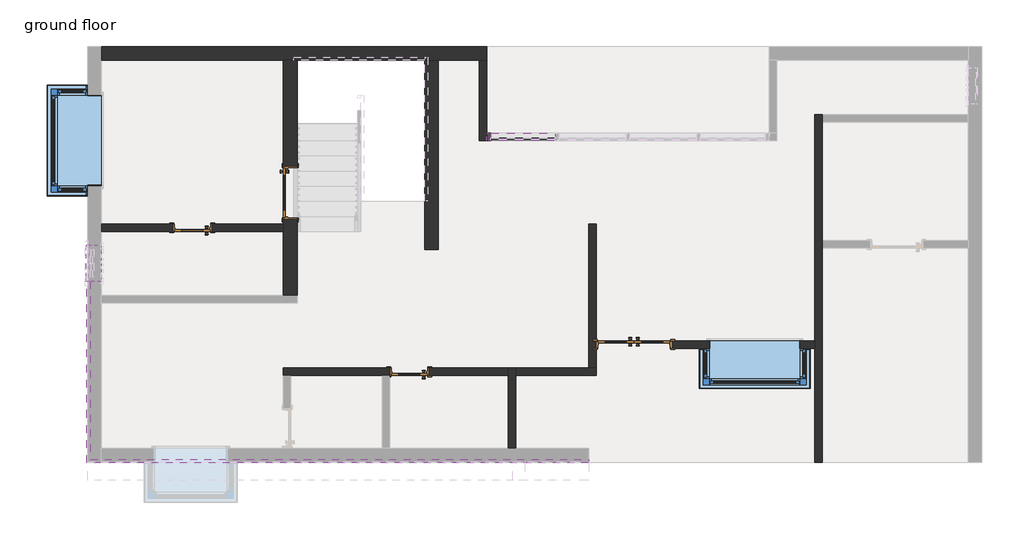
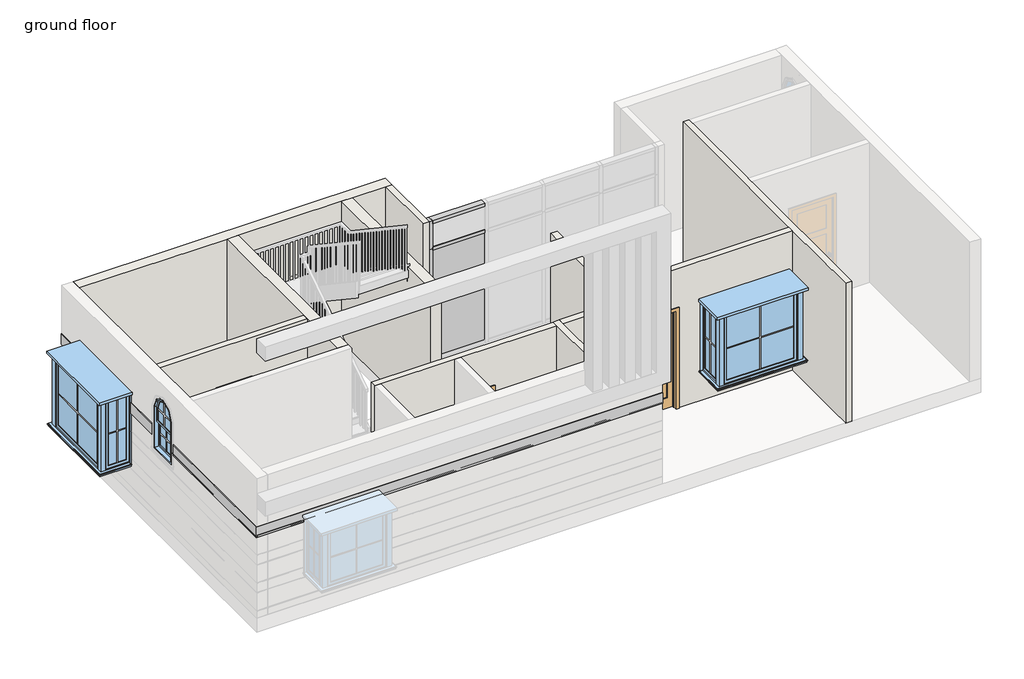
# One storey, part 3 of 5: 11 walls, 4 doors, 4 members, 3 windows, 1 plate, 1 proxy.
"""IFC4 building model written with IfcOpenShell, lengths in millimetres."""

from ifc_helpers import new_model, si_unit, frame, origin, place, context, project, spatial, polyline, circle_curve, ellipse_curve, outline, extrude, faceted_brep, transform, mapped, element, save
from ifc_brep_helpers import plane_surface, cylinder_surface, revolved_surface, advanced_brep
from components import door_interior_double_full_glass_wood_double_door_4_x_7_060eee9d, door_596d7c92, door_5abea521, member_ee409385, member_47bfaf8a, member_5474ae84, member_0cc0e230, system_panel_glazed_91cb7ab6, window_153fc52c, window_dda79932, window_777a1d98

model = new_model("IFC4")

# Units and contexts
model_context = context("Model", 3, world=origin())
ifc_project = project(units=[si_unit("LENGTHUNIT", "METRE", prefix="MILLI")], contexts=[model_context])

# Site, building, storey
site = spatial("IfcSite", under=ifc_project)
building = spatial("IfcBuilding", under=site)
storey = spatial("IfcBuildingStorey", under=building, Name="ground floor", Elevation=304.8)

# Proxy
placement = place(None, origin())
element("IfcBuildingElementProxy", 1, Name="Reveal", ObjectType="Reveal", at=placement, inside=storey, context=model_context, shape_type="AdvancedBrep", body=[
    advanced_brep(
    [(-13193.9516301, -7280.1146427, 2298.7), (-13130.7056301, -7216.8686427, 2298.7), (-13130.7056301, -7216.8686427, 2297.3203242), (-13135.0884393, -7221.2514519, 2292.1465897), (-13158.7091301, -7244.8721427, 2288.2098), (-13177.9470117, -7264.1100243, 2285.00348), (-13186.7126301, -7272.8756427, 2274.656011), (-13186.7126301, -7272.8756427, 2094.143989), (-13177.9470117, -7264.1100243, 2083.79652), (-13158.7091301, -7244.8721427, 2080.5902), (-13135.0884393, -7221.2514519, 2076.6534103), (-13130.7056301, -7216.8686427, 2071.4796758), (-13130.7056301, -7216.8686427, 2070.1), (-13193.9516301, -7280.1146427, 2070.1), (-4797.0672301, -7280.1146427, 2298.7), (-4797.0672301, -7280.1146427, 2070.1), (-4797.0672301, -7216.8686427, 2070.1), (-4797.0672301, -7216.8686427, 2071.4796758), (-4797.0672301, -7221.2514519, 2076.6534103), (-4797.0672301, -7244.8721427, 2080.5902), (-4797.0672301, -7264.1100243, 2083.79652), (-4797.0672301, -7272.8756427, 2094.143989), (-4797.0672301, -7272.8756427, 2274.656011), (-4797.0672301, -7264.1100243, 2285.00348), (-4797.0672301, -7244.8721427, 2288.2098), (-4797.0672301, -7221.2514519, 2292.1465897), (-4797.0672301, -7216.8686427, 2297.3203242), (-4797.0672301, -7216.8686427, 2298.7)],
    [
        (0, 1),
        (1, 2),
        (2, 3, ellipse_curve(frame((-13135.9507301, -7222.1137427, 2297.3203242), z_axis=(-0.7071067811865476, 0.7071067811865476, 0.0), x_axis=(-0.7071067811865475, -0.7071067811865476, 0.0)), 7.4176916, 5.2451)),
        (3, 4),
        (4, 5),
        (5, 6, ellipse_curve(frame((-13176.2224301, -7262.3854427, 2274.656011), z_axis=(0.7071067811865476, -0.7071067811865476, 0.0), x_axis=(0.7071067811865475, 0.7071067811865476, 0.0)), 14.8353831, 10.4902)),
        (6, 7),
        (7, 8, ellipse_curve(frame((-13176.2224301, -7262.3854427, 2094.143989), z_axis=(0.7071067811865476, -0.7071067811865476, 0.0), x_axis=(0.7071067811865475, 0.7071067811865476, 0.0)), 14.8353831, 10.4902)),
        (8, 9),
        (9, 10),
        (10, 11, ellipse_curve(frame((-13135.9507301, -7222.1137427, 2071.4796758), z_axis=(-0.7071067811865476, 0.7071067811865476, 0.0), x_axis=(-0.7071067811865475, -0.7071067811865476, 0.0)), 7.4176916, 5.2451)),
        (11, 12),
        (12, 13),
        (13, 0),
        (14, 15),
        (15, 16),
        (16, 17),
        (17, 18, circle_curve(frame((-4797.0672301, -7222.1137427, 2071.4796758), z_axis=(1.0, 0.0, 0.0), x_axis=(0.0, 1.0, 0.0)), 5.2451)),
        (18, 19),
        (19, 20),
        (20, 21, circle_curve(frame((-4797.0672301, -7262.3854427, 2094.143989), z_axis=(-1.0, 0.0, 0.0), x_axis=(0.0, 1.0, 0.0)), 10.4902)),
        (21, 22),
        (22, 23, circle_curve(frame((-4797.0672301, -7262.3854427, 2274.656011), z_axis=(-1.0, 0.0, 0.0), x_axis=(0.0, 1.0, 0.0)), 10.4902)),
        (23, 24),
        (24, 25),
        (25, 26, circle_curve(frame((-4797.0672301, -7222.1137427, 2297.3203242), z_axis=(1.0, 0.0, 0.0), x_axis=(0.0, 1.0, 0.0)), 5.2451)),
        (26, 27),
        (27, 14),
        (0, 14),
        (27, 1),
        (26, 2),
        (25, 3),
        (24, 4),
        (23, 5),
        (22, 6),
        (21, 7),
        (20, 8),
        (19, 9),
        (18, 10),
        (17, 11),
        (16, 12),
        (15, 13),
    ],
    [
        plane_surface(frame((-13179.0672301, -7265.2302427, 1879.6), z_axis=(-0.7071067811865476, 0.7071067811865476, 0.0), x_axis=(0.7071067811865476, 0.7071067811865476, 0.0))),
        plane_surface(frame((-4797.0672301, -7265.2302427, 2060.2898298), z_axis=(1.0, 0.0, 0.0), x_axis=(0.0, 1.0, 0.0))),
        plane_surface(frame((-13193.9516301, -7280.1146427, 2298.7), z_axis=(0.0, 0.0, 1.0), x_axis=(1.0, 0.0, 0.0))),
        plane_surface(frame((-13130.7056301, -7216.8686427, 2298.7), z_axis=(0.0, 1.0, 0.0), x_axis=(1.0, 0.0, 0.0))),
        cylinder_surface(frame((-13179.0672301, -7222.1137427, 2297.3203242), z_axis=(-1.0, 0.0, 0.0), x_axis=(0.0, 1.0, 0.0)), 5.2451),
        plane_surface(frame((-13135.0884393, -7221.2514519, 2292.1465897), z_axis=(0.0, 0.16439930721687082, -0.9863938705135049), x_axis=(1.0, 0.0, 0.0))),
        plane_surface(frame((-13158.7091301, -7244.8721427, 2288.2098), z_axis=(0.0, 0.16439930721687146, -0.9863938705135048), x_axis=(1.0, 0.0, 0.0))),
        revolved_surface(polyline([(-4797.0672300999995, -7251.8952426999995, 2274.656011), (-13186.7126301, -7251.8952426999995, 2274.656011)]), (-13179.0672301, -7262.3854427, 2274.656011), (1.0, 0.0, 0.0)),
        plane_surface(frame((-13186.7126301, -7272.8756427, 2274.656011), z_axis=(0.0, 1.0, 0.0), x_axis=(1.0, 0.0, 0.0))),
        revolved_surface(polyline([(-4797.0672300999995, -7251.8952426999995, 2094.143989), (-13186.7126301, -7251.8952426999995, 2094.143989)]), (-13179.0672301, -7262.3854427, 2094.143989), (1.0, 0.0, 0.0)),
        plane_surface(frame((-13177.9470117, -7264.1100243, 2083.79652), z_axis=(0.0, 0.1643993072168769, 0.9863938705135039), x_axis=(1.0, 0.0, 0.0))),
        plane_surface(frame((-13158.7091301, -7244.8721427, 2080.5902), z_axis=(0.0, 0.16439930721687793, 0.9863938705135037), x_axis=(1.0, 0.0, 0.0))),
        cylinder_surface(frame((-13179.0672301, -7222.1137427, 2071.4796758), z_axis=(-1.0, 0.0, 0.0), x_axis=(0.0, 1.0, 0.0)), 5.2451),
        plane_surface(frame((-13130.7056301, -7216.8686427, 2071.4796758), z_axis=(0.0, 1.0, 0.0), x_axis=(1.0, 0.0, 0.0))),
        plane_surface(frame((-13130.7056301, -7216.8686427, 2070.1), z_axis=(0.0, 0.0, -1.0), x_axis=(1.0, 0.0, 0.0))),
        plane_surface(frame((-13193.9516301, -7280.1146427, 2070.1), z_axis=(0.0, -1.0, 0.0), x_axis=(1.0, 0.0, 0.0))),
    ],
    [
        (0, [[1, 2, 3, 4, 5, 6, 7, 8, 9, 10, 11, 12, 13, 14]]),
        (1, [[15, 16, 17, 18, 19, 20, 21, 22, 23, 24, 25, 26, 27, 28]]),
        (2, [[-1, 29, -28, 30]]),
        (3, [[-2, -30, -27, 31]]),
        (4, [[-3, -31, -26, 32]]),
        (5, [[-4, -32, -25, 33]]),
        (6, [[-5, -33, -24, 34]]),
        (7, [[-6, -34, -23, 35]]),
        (8, [[-7, -35, -22, 36]]),
        (9, [[-8, -36, -21, 37]]),
        (10, [[-9, -37, -20, 38]]),
        (11, [[-10, -38, -19, 39]]),
        (12, [[-11, -39, -18, 40]]),
        (13, [[-12, -40, -17, 41]]),
        (14, [[-13, -41, -16, 42]]),
        (15, [[-14, -42, -15, -29]]),
    ],
),
    advanced_brep(
    [(-13193.9516301, -4242.6302427, 2298.7), (-13130.7056301, -4242.6302427, 2298.7), (-13130.7056301, -4242.6302427, 2297.3203242), (-13135.0884393, -4242.6302427, 2292.1465897), (-13158.7091301, -4242.6302427, 2288.2098), (-13177.9470117, -4242.6302427, 2285.00348), (-13186.7126301, -4242.6302427, 2274.656011), (-13186.7126301, -4242.6302427, 2094.143989), (-13177.9470117, -4242.6302427, 2083.79652), (-13158.7091301, -4242.6302427, 2080.5902), (-13135.0884393, -4242.6302427, 2076.6534103), (-13130.7056301, -4242.6302427, 2071.4796758), (-13130.7056301, -4242.6302427, 2070.1), (-13193.9516301, -4242.6302427, 2070.1), (-13193.9516301, -7280.1146427, 2298.7), (-13193.9516301, -7280.1146427, 2070.1), (-13130.7056301, -7216.8686427, 2070.1), (-13130.7056301, -7216.8686427, 2071.4796758), (-13135.0884393, -7221.2514519, 2076.6534103), (-13158.7091301, -7244.8721427, 2080.5902), (-13177.9470117, -7264.1100243, 2083.79652), (-13186.7126301, -7272.8756427, 2094.143989), (-13186.7126301, -7272.8756427, 2274.656011), (-13177.9470117, -7264.1100243, 2285.00348), (-13158.7091301, -7244.8721427, 2288.2098), (-13135.0884393, -7221.2514519, 2292.1465897), (-13130.7056301, -7216.8686427, 2297.3203242), (-13130.7056301, -7216.8686427, 2298.7)],
    [
        (0, 1),
        (1, 2),
        (2, 3, circle_curve(frame((-13135.9507301, -4242.6302427, 2297.3203242), z_axis=(0.0, 1.0, 0.0), x_axis=(1.0, 0.0, 0.0)), 5.2451)),
        (3, 4),
        (4, 5),
        (5, 6, circle_curve(frame((-13176.2224301, -4242.6302427, 2274.656011), z_axis=(0.0, -1.0, 0.0), x_axis=(1.0, 0.0, 0.0)), 10.4902)),
        (6, 7),
        (7, 8, circle_curve(frame((-13176.2224301, -4242.6302427, 2094.143989), z_axis=(0.0, -1.0, 0.0), x_axis=(1.0, 0.0, 0.0)), 10.4902)),
        (8, 9),
        (9, 10),
        (10, 11, circle_curve(frame((-13135.9507301, -4242.6302427, 2071.4796758), z_axis=(0.0, 1.0, 0.0), x_axis=(1.0, 0.0, 0.0)), 5.2451)),
        (11, 12),
        (12, 13),
        (13, 0),
        (14, 15),
        (15, 16),
        (16, 17),
        (17, 18, ellipse_curve(frame((-13135.9507301, -7222.1137427, 2071.4796758), z_axis=(0.7071067811865476, -0.7071067811865476, 0.0), x_axis=(0.7071067811865477, 0.7071067811865474, 0.0)), 7.4176916, 5.2451)),
        (18, 19),
        (19, 20),
        (20, 21, ellipse_curve(frame((-13176.2224301, -7262.3854427, 2094.143989), z_axis=(-0.7071067811865476, 0.7071067811865476, 0.0), x_axis=(-0.7071067811865477, -0.7071067811865474, 0.0)), 14.8353831, 10.4902)),
        (21, 22),
        (22, 23, ellipse_curve(frame((-13176.2224301, -7262.3854427, 2274.656011), z_axis=(-0.7071067811865476, 0.7071067811865476, 0.0), x_axis=(-0.7071067811865477, -0.7071067811865474, 0.0)), 14.8353831, 10.4902)),
        (23, 24),
        (24, 25),
        (25, 26, ellipse_curve(frame((-13135.9507301, -7222.1137427, 2297.3203242), z_axis=(0.7071067811865476, -0.7071067811865476, 0.0), x_axis=(0.7071067811865477, 0.7071067811865474, 0.0)), 7.4176916, 5.2451)),
        (26, 27),
        (27, 14),
        (0, 14),
        (27, 1),
        (26, 2),
        (25, 3),
        (24, 4),
        (23, 5),
        (22, 6),
        (21, 7),
        (20, 8),
        (19, 9),
        (18, 10),
        (17, 11),
        (16, 12),
        (15, 13),
    ],
    [
        plane_surface(frame((-13179.0672301, -4242.6302427, 2743.2), z_axis=(0.0, 1.0, 0.0), x_axis=(1.0, 0.0, 0.0))),
        plane_surface(frame((-13179.0672301, -7265.2302427, 1879.6), z_axis=(0.7071067811865476, -0.7071067811865476, 0.0), x_axis=(0.7071067811865476, 0.7071067811865476, 0.0))),
        plane_surface(frame((-13193.9516301, -4242.6302427, 2298.7), z_axis=(0.0, 0.0, 1.0), x_axis=(0.0, -1.0, 0.0))),
        plane_surface(frame((-13130.7056301, -4242.6302427, 2298.7), z_axis=(1.0, 0.0, 0.0), x_axis=(0.0, -1.0, 0.0))),
        cylinder_surface(frame((-13135.9507301, -4242.6302427, 2297.3203242), z_axis=(0.0, 1.0, 0.0), x_axis=(1.0, 0.0, 0.0)), 5.2451),
        plane_surface(frame((-13135.0884393, -4242.6302427, 2292.1465897), z_axis=(0.16439930721687082, 0.0, -0.9863938705135049), x_axis=(0.0, -1.0, 0.0))),
        plane_surface(frame((-13158.7091301, -4242.6302427, 2288.2098), z_axis=(0.16439930721687146, 0.0, -0.9863938705135048), x_axis=(0.0, -1.0, 0.0))),
        revolved_surface(polyline([(-13165.7322301, -7272.8756427, 2274.656011), (-13165.7322301, -4242.6302427, 2274.656011)]), (-13176.2224301, -4242.6302427, 2274.656011), (0.0, -1.0, 0.0)),
        plane_surface(frame((-13186.7126301, -4242.6302427, 2274.656011), z_axis=(1.0, 0.0, 0.0), x_axis=(0.0, -1.0, 0.0))),
        revolved_surface(polyline([(-13165.7322301, -7272.8756427, 2094.143989), (-13165.7322301, -4242.6302427, 2094.143989)]), (-13176.2224301, -4242.6302427, 2094.143989), (0.0, -1.0, 0.0)),
        plane_surface(frame((-13177.9470117, -4242.6302427, 2083.79652), z_axis=(0.1643993072168769, 0.0, 0.9863938705135039), x_axis=(0.0, -1.0, 0.0))),
        plane_surface(frame((-13158.7091301, -4242.6302427, 2080.5902), z_axis=(0.16439930721687793, 0.0, 0.9863938705135037), x_axis=(0.0, -1.0, 0.0))),
        cylinder_surface(frame((-13135.9507301, -4242.6302427, 2071.4796758), z_axis=(0.0, 1.0, 0.0), x_axis=(1.0, 0.0, 0.0)), 5.2451),
        plane_surface(frame((-13130.7056301, -4242.6302427, 2071.4796758), z_axis=(1.0, 0.0, 0.0), x_axis=(0.0, -1.0, 0.0))),
        plane_surface(frame((-13130.7056301, -4242.6302427, 2070.1), z_axis=(0.0, 0.0, -1.0), x_axis=(0.0, -1.0, 0.0))),
        plane_surface(frame((-13193.9516301, -4242.6302427, 2070.1), z_axis=(-1.0, 0.0, 0.0), x_axis=(0.0, -1.0, 0.0))),
    ],
    [
        (0, [[1, 2, 3, 4, 5, 6, 7, 8, 9, 10, 11, 12, 13, 14]]),
        (1, [[15, 16, 17, 18, 19, 20, 21, 22, 23, 24, 25, 26, 27, 28]]),
        (2, [[-1, 29, -28, 30]]),
        (3, [[-2, -30, -27, 31]]),
        (4, [[-3, -31, -26, 32]]),
        (5, [[-4, -32, -25, 33]]),
        (6, [[-5, -33, -24, 34]]),
        (7, [[-6, -34, -23, 35]]),
        (8, [[-7, -35, -22, 36]]),
        (9, [[-8, -36, -21, 37]]),
        (10, [[-9, -37, -20, 38]]),
        (11, [[-10, -38, -19, 39]]),
        (12, [[-11, -39, -18, 40]]),
        (13, [[-12, -40, -17, 41]]),
        (14, [[-13, -41, -16, 42]]),
        (15, [[-14, -42, -15, -29]]),
    ],
),
    advanced_brep(
    [(-13193.9516301, -2642.4302427, 2298.7), (-13130.7056301, -2642.4302427, 2298.7), (-13130.7056301, -2642.4302427, 2297.3203242), (-13135.0884393, -2642.4302427, 2292.1465897), (-13158.7091301, -2642.4302427, 2288.2098), (-13177.9470117, -2642.4302427, 2285.00348), (-13186.7126301, -2642.4302427, 2274.656011), (-13186.7126301, -2642.4302427, 2094.143989), (-13177.9470117, -2642.4302427, 2083.79652), (-13158.7091301, -2642.4302427, 2080.5902), (-13135.0884393, -2642.4302427, 2076.6534103), (-13130.7056301, -2642.4302427, 2071.4796758), (-13130.7056301, -2642.4302427, 2070.1), (-13193.9516301, -2642.4302427, 2070.1), (-13193.9516301, -3633.0302427, 2298.7), (-13193.9516301, -3633.0302427, 2070.1), (-13130.7056301, -3633.0302427, 2070.1), (-13130.7056301, -3633.0302427, 2071.4796758), (-13135.0884393, -3633.0302427, 2076.6534103), (-13158.7091301, -3633.0302427, 2080.5902), (-13177.9470117, -3633.0302427, 2083.79652), (-13186.7126301, -3633.0302427, 2094.143989), (-13186.7126301, -3633.0302427, 2274.656011), (-13177.9470117, -3633.0302427, 2285.00348), (-13158.7091301, -3633.0302427, 2288.2098), (-13135.0884393, -3633.0302427, 2292.1465897), (-13130.7056301, -3633.0302427, 2297.3203242), (-13130.7056301, -3633.0302427, 2298.7)],
    [
        (0, 1),
        (1, 2),
        (2, 3, circle_curve(frame((-13135.9507301, -2642.4302427, 2297.3203242), z_axis=(0.0, 1.0, 0.0), x_axis=(1.0, 0.0, 0.0)), 5.2451)),
        (3, 4),
        (4, 5),
        (5, 6, circle_curve(frame((-13176.2224301, -2642.4302427, 2274.656011), z_axis=(0.0, -1.0, 0.0), x_axis=(1.0, 0.0, 0.0)), 10.4902)),
        (6, 7),
        (7, 8, circle_curve(frame((-13176.2224301, -2642.4302427, 2094.143989), z_axis=(0.0, -1.0, 0.0), x_axis=(1.0, 0.0, 0.0)), 10.4902)),
        (8, 9),
        (9, 10),
        (10, 11, circle_curve(frame((-13135.9507301, -2642.4302427, 2071.4796758), z_axis=(0.0, 1.0, 0.0), x_axis=(1.0, 0.0, 0.0)), 5.2451)),
        (11, 12),
        (12, 13),
        (13, 0),
        (14, 15),
        (15, 16),
        (16, 17),
        (17, 18, circle_curve(frame((-13135.9507301, -3633.0302427, 2071.4796758), z_axis=(0.0, -1.0, 0.0), x_axis=(1.0, 0.0, 0.0)), 5.2451)),
        (18, 19),
        (19, 20),
        (20, 21, circle_curve(frame((-13176.2224301, -3633.0302427, 2094.143989), z_axis=(0.0, 1.0, 0.0), x_axis=(1.0, 0.0, 0.0)), 10.4902)),
        (21, 22),
        (22, 23, circle_curve(frame((-13176.2224301, -3633.0302427, 2274.656011), z_axis=(0.0, 1.0, 0.0), x_axis=(1.0, 0.0, 0.0)), 10.4902)),
        (23, 24),
        (24, 25),
        (25, 26, circle_curve(frame((-13135.9507301, -3633.0302427, 2297.3203242), z_axis=(0.0, -1.0, 0.0), x_axis=(1.0, 0.0, 0.0)), 5.2451)),
        (26, 27),
        (27, 14),
        (0, 14),
        (27, 1),
        (26, 2),
        (25, 3),
        (24, 4),
        (23, 5),
        (22, 6),
        (21, 7),
        (20, 8),
        (19, 9),
        (18, 10),
        (17, 11),
        (16, 12),
        (15, 13),
    ],
    [
        plane_surface(frame((-12950.4672301, -2642.4302427, 914.4), z_axis=(0.0, 1.0, 0.0), x_axis=(-1.0, 0.0, 0.0))),
        plane_surface(frame((-13179.0672301, -3633.0302427, 1828.8), z_axis=(0.0, -1.0, 0.0), x_axis=(1.0, 0.0, 0.0))),
        plane_surface(frame((-13193.9516301, -2642.4302427, 2298.7), z_axis=(0.0, 0.0, 1.0), x_axis=(0.0, -1.0, 0.0))),
        plane_surface(frame((-13130.7056301, -2642.4302427, 2298.7), z_axis=(1.0, 0.0, 0.0), x_axis=(0.0, -1.0, 0.0))),
        cylinder_surface(frame((-13135.9507301, -2642.4302427, 2297.3203242), z_axis=(0.0, 1.0, 0.0), x_axis=(1.0, 0.0, 0.0)), 5.2451),
        plane_surface(frame((-13135.0884393, -2642.4302427, 2292.1465897), z_axis=(0.16439930721687082, 0.0, -0.9863938705135049), x_axis=(0.0, -1.0, 0.0))),
        plane_surface(frame((-13158.7091301, -2642.4302427, 2288.2098), z_axis=(0.16439930721687146, 0.0, -0.9863938705135048), x_axis=(0.0, -1.0, 0.0))),
        revolved_surface(polyline([(-13165.7322301, -3633.0302427, 2274.656011), (-13165.7322301, -2642.4302427, 2274.656011)]), (-13176.2224301, -2642.4302427, 2274.656011), (0.0, -1.0, 0.0)),
        plane_surface(frame((-13186.7126301, -2642.4302427, 2274.656011), z_axis=(1.0, 0.0, 0.0), x_axis=(0.0, -1.0, 0.0))),
        revolved_surface(polyline([(-13165.7322301, -3633.0302427, 2094.143989), (-13165.7322301, -2642.4302427, 2094.143989)]), (-13176.2224301, -2642.4302427, 2094.143989), (0.0, -1.0, 0.0)),
        plane_surface(frame((-13177.9470117, -2642.4302427, 2083.79652), z_axis=(0.1643993072168769, 0.0, 0.9863938705135039), x_axis=(0.0, -1.0, 0.0))),
        plane_surface(frame((-13158.7091301, -2642.4302427, 2080.5902), z_axis=(0.16439930721687793, 0.0, 0.9863938705135037), x_axis=(0.0, -1.0, 0.0))),
        cylinder_surface(frame((-13135.9507301, -2642.4302427, 2071.4796758), z_axis=(0.0, 1.0, 0.0), x_axis=(1.0, 0.0, 0.0)), 5.2451),
        plane_surface(frame((-13130.7056301, -2642.4302427, 2071.4796758), z_axis=(1.0, 0.0, 0.0), x_axis=(0.0, -1.0, 0.0))),
        plane_surface(frame((-13130.7056301, -2642.4302427, 2070.1), z_axis=(0.0, 0.0, -1.0), x_axis=(0.0, -1.0, 0.0))),
        plane_surface(frame((-13193.9516301, -2642.4302427, 2070.1), z_axis=(-1.0, 0.0, 0.0), x_axis=(0.0, -1.0, 0.0))),
    ],
    [
        (0, [[1, 2, 3, 4, 5, 6, 7, 8, 9, 10, 11, 12, 13, 14]]),
        (1, [[15, 16, 17, 18, 19, 20, 21, 22, 23, 24, 25, 26, 27, 28]]),
        (2, [[-1, 29, -28, 30]]),
        (3, [[-2, -30, -27, 31]]),
        (4, [[-3, -31, -26, 32]]),
        (5, [[-4, -32, -25, 33]]),
        (6, [[-5, -33, -24, 34]]),
        (7, [[-6, -34, -23, 35]]),
        (8, [[-7, -35, -22, 36]]),
        (9, [[-8, -36, -21, 37]]),
        (10, [[-9, -37, -20, 38]]),
        (11, [[-10, -38, -19, 39]]),
        (12, [[-11, -39, -18, 40]]),
        (13, [[-12, -40, -17, 41]]),
        (14, [[-13, -41, -16, 42]]),
        (15, [[-14, -42, -15, -29]]),
    ],
),
    advanced_brep(
    [(-13193.9516301, -305.6302427, 2298.7), (-13130.7056301, -305.6302427, 2298.7), (-13130.7056301, -305.6302427, 2297.3203242), (-13135.0884393, -305.6302427, 2292.1465897), (-13158.7091301, -305.6302427, 2288.2098), (-13177.9470117, -305.6302427, 2285.00348), (-13186.7126301, -305.6302427, 2274.656011), (-13186.7126301, -305.6302427, 2094.143989), (-13177.9470117, -305.6302427, 2083.79652), (-13158.7091301, -305.6302427, 2080.5902), (-13135.0884393, -305.6302427, 2076.6534103), (-13130.7056301, -305.6302427, 2071.4796758), (-13130.7056301, -305.6302427, 2070.1), (-13193.9516301, -305.6302427, 2070.1), (-13193.9516301, -1118.4302427, 2298.7), (-13193.9516301, -1118.4302427, 2070.1), (-13130.7056301, -1118.4302427, 2070.1), (-13130.7056301, -1118.4302427, 2071.4796758), (-13135.0884393, -1118.4302427, 2076.6534103), (-13158.7091301, -1118.4302427, 2080.5902), (-13177.9470117, -1118.4302427, 2083.79652), (-13186.7126301, -1118.4302427, 2094.143989), (-13186.7126301, -1118.4302427, 2274.656011), (-13177.9470117, -1118.4302427, 2285.00348), (-13158.7091301, -1118.4302427, 2288.2098), (-13135.0884393, -1118.4302427, 2292.1465897), (-13130.7056301, -1118.4302427, 2297.3203242), (-13130.7056301, -1118.4302427, 2298.7)],
    [
        (0, 1),
        (1, 2),
        (2, 3, circle_curve(frame((-13135.9507301, -305.6302427, 2297.3203242), z_axis=(0.0, 1.0, 0.0), x_axis=(1.0, 0.0, 0.0)), 5.2451)),
        (3, 4),
        (4, 5),
        (5, 6, circle_curve(frame((-13176.2224301, -305.6302427, 2274.656011), z_axis=(0.0, -1.0, 0.0), x_axis=(1.0, 0.0, 0.0)), 10.4902)),
        (6, 7),
        (7, 8, circle_curve(frame((-13176.2224301, -305.6302427, 2094.143989), z_axis=(0.0, -1.0, 0.0), x_axis=(1.0, 0.0, 0.0)), 10.4902)),
        (8, 9),
        (9, 10),
        (10, 11, circle_curve(frame((-13135.9507301, -305.6302427, 2071.4796758), z_axis=(0.0, 1.0, 0.0), x_axis=(1.0, 0.0, 0.0)), 5.2451)),
        (11, 12),
        (12, 13),
        (13, 0),
        (14, 15),
        (15, 16),
        (16, 17),
        (17, 18, circle_curve(frame((-13135.9507301, -1118.4302427, 2071.4796758), z_axis=(0.0, -1.0, 0.0), x_axis=(1.0, 0.0, 0.0)), 5.2451)),
        (18, 19),
        (19, 20),
        (20, 21, circle_curve(frame((-13176.2224301, -1118.4302427, 2094.143989), z_axis=(0.0, 1.0, 0.0), x_axis=(1.0, 0.0, 0.0)), 10.4902)),
        (21, 22),
        (22, 23, circle_curve(frame((-13176.2224301, -1118.4302427, 2274.656011), z_axis=(0.0, 1.0, 0.0), x_axis=(1.0, 0.0, 0.0)), 10.4902)),
        (23, 24),
        (24, 25),
        (25, 26, circle_curve(frame((-13135.9507301, -1118.4302427, 2297.3203242), z_axis=(0.0, -1.0, 0.0), x_axis=(1.0, 0.0, 0.0)), 5.2451)),
        (26, 27),
        (27, 14),
        (0, 14),
        (27, 1),
        (26, 2),
        (25, 3),
        (24, 4),
        (23, 5),
        (22, 6),
        (21, 7),
        (20, 8),
        (19, 9),
        (18, 10),
        (17, 11),
        (16, 12),
        (15, 13),
    ],
    [
        plane_surface(frame((-12942.6830845, -305.6302427, 304.8), z_axis=(0.0, 1.0, 0.0), x_axis=(-1.0, 0.0, 0.0))),
        plane_surface(frame((-12950.4672301, -1118.4302427, 2489.2), z_axis=(0.0, -1.0, 0.0), x_axis=(-1.0, 0.0, 0.0))),
        plane_surface(frame((-13193.9516301, -305.6302427, 2298.7), z_axis=(0.0, 0.0, 1.0), x_axis=(0.0, -1.0, 0.0))),
        plane_surface(frame((-13130.7056301, -305.6302427, 2298.7), z_axis=(1.0, 0.0, 0.0), x_axis=(0.0, -1.0, 0.0))),
        cylinder_surface(frame((-13135.9507301, -305.6302427, 2297.3203242), z_axis=(0.0, 1.0, 0.0), x_axis=(1.0, 0.0, 0.0)), 5.2451),
        plane_surface(frame((-13135.0884393, -305.6302427, 2292.1465897), z_axis=(0.16439930721687082, 0.0, -0.9863938705135049), x_axis=(0.0, -1.0, 0.0))),
        plane_surface(frame((-13158.7091301, -305.6302427, 2288.2098), z_axis=(0.16439930721687146, 0.0, -0.9863938705135048), x_axis=(0.0, -1.0, 0.0))),
        revolved_surface(polyline([(-13165.7322301, -1118.4302427, 2274.656011), (-13165.7322301, -305.6302427, 2274.656011)]), (-13176.2224301, -305.6302427, 2274.656011), (0.0, -1.0, 0.0)),
        plane_surface(frame((-13186.7126301, -305.6302427, 2274.656011), z_axis=(1.0, 0.0, 0.0), x_axis=(0.0, -1.0, 0.0))),
        revolved_surface(polyline([(-13165.7322301, -1118.4302427, 2094.143989), (-13165.7322301, -305.6302427, 2094.143989)]), (-13176.2224301, -305.6302427, 2094.143989), (0.0, -1.0, 0.0)),
        plane_surface(frame((-13177.9470117, -305.6302427, 2083.79652), z_axis=(0.1643993072168769, 0.0, 0.9863938705135039), x_axis=(0.0, -1.0, 0.0))),
        plane_surface(frame((-13158.7091301, -305.6302427, 2080.5902), z_axis=(0.16439930721687793, 0.0, 0.9863938705135037), x_axis=(0.0, -1.0, 0.0))),
        cylinder_surface(frame((-13135.9507301, -305.6302427, 2071.4796758), z_axis=(0.0, 1.0, 0.0), x_axis=(1.0, 0.0, 0.0)), 5.2451),
        plane_surface(frame((-13130.7056301, -305.6302427, 2071.4796758), z_axis=(1.0, 0.0, 0.0), x_axis=(0.0, -1.0, 0.0))),
        plane_surface(frame((-13130.7056301, -305.6302427, 2070.1), z_axis=(0.0, 0.0, -1.0), x_axis=(0.0, -1.0, 0.0))),
        plane_surface(frame((-13193.9516301, -305.6302427, 2070.1), z_axis=(-1.0, 0.0, 0.0), x_axis=(0.0, -1.0, 0.0))),
    ],
    [
        (0, [[1, 2, 3, 4, 5, 6, 7, 8, 9, 10, 11, 12, 13, 14]]),
        (1, [[15, 16, 17, 18, 19, 20, 21, 22, 23, 24, 25, 26, 27, 28]]),
        (2, [[-1, 29, -28, 30]]),
        (3, [[-2, -30, -27, 31]]),
        (4, [[-3, -31, -26, 32]]),
        (5, [[-4, -32, -25, 33]]),
        (6, [[-5, -33, -24, 34]]),
        (7, [[-6, -34, -23, 35]]),
        (8, [[-7, -35, -22, 36]]),
        (9, [[-8, -36, -21, 37]]),
        (10, [[-9, -37, -20, 38]]),
        (11, [[-10, -38, -19, 39]]),
        (12, [[-11, -39, -18, 40]]),
        (13, [[-12, -40, -17, 41]]),
        (14, [[-13, -41, -16, 42]]),
        (15, [[-14, -42, -15, -29]]),
    ],
),
])

# Doors
door_interior_double_full_glass_wood_double_door_4_x_7_shape = door_interior_double_full_glass_wood_double_door_4_x_7_060eee9d(model_context)
element("IfcDoor", 2, ObjectType="Door-Interior-Double-Full Glass-Wood : DOUBLE DOOR 4' X 7'", at=placement, inside=storey, context=model_context, shape_type="MappedRepresentation", body=[
    mapped(door_interior_double_full_glass_wood_double_door_4_x_7_shape, transform((-4035.0672301, -5293.5552427, 304.8), x_axis=(1.0, 0.0, 0.0), y_axis=(0.0, 1.0, 0.0), z_axis=(0.0, 0.0, 1.0))),
])
door_shape = door_596d7c92(model_context)
element("IfcDoor", 3, ObjectType="Door-Interior-Single-2_Panel-Wood : 24\" x 84\"", at=placement, inside=storey, context=model_context, shape_type="MappedRepresentation", body=[
    mapped(door_shape, transform((-11426.4672301, -3344.1052427, 304.8), x_axis=(-1.0, 0.0, 0.0), y_axis=(0.0, -1.0, 0.0), z_axis=(0.0, 0.0, 1.0))),
])
element("IfcDoor", 4, ObjectType="Door-Interior-Single-2_Panel-Wood : 24\" x 84\"", at=placement, inside=storey, context=model_context, shape_type="MappedRepresentation", body=[
    mapped(door_shape, transform((-7794.2672301, -5757.1052427, 304.8), x_axis=(-1.0, 0.0, 0.0), y_axis=(0.0, -1.0, 0.0), z_axis=(0.0, 0.0, 1.0))),
])
door_2_shape = door_5abea521(model_context)
element("IfcDoor", 5, ObjectType="Door-Interior-Single-3_Panel_Vert-Wood : 33\" x 84\"", at=placement, inside=storey, context=model_context, shape_type="MappedRepresentation", body=[
    mapped(door_2_shape, transform((-9791.3422301, -2756.7302427, 304.8), x_axis=(0.0, -1.0, 0.0), y_axis=(1.0, 0.0, 0.0), z_axis=(0.0, 0.0, 1.0))),
])

# Members
member_shape = member_ee409385(model_context)
element("IfcMember", 6, ObjectType="Rectangular Mullion : 2.5\" x 5\" rectangular", at=placement, inside=storey, context=model_context, shape_type="MappedRepresentation", body=[
    mapped(member_shape, transform((-6498.8672301, -1816.9302427, 304.8), x_axis=(-1.0, 0.0, 0.0), y_axis=(0.0, 1.0, 0.0), z_axis=(0.0, 0.0, -1.0))),
])
member_2_shape = member_47bfaf8a(model_context)
element("IfcMember", 7, ObjectType="Rectangular Mullion : 2.5\" x 5\" rectangular", at=placement, inside=storey, context=model_context, shape_type="MappedRepresentation", body=[
    mapped(member_2_shape, transform((-6498.8672301, -1816.9302427, 2743.2), x_axis=(-1.0, 0.0, 0.0), y_axis=(0.0, 1.0, 0.0), z_axis=(0.0, 0.0, -1.0))),
])
member_3_shape = member_5474ae84(model_context)
element("IfcMember", 8, ObjectType="Rectangular Mullion : 2.5\" x 5\" rectangular", at=placement, inside=storey, context=model_context, shape_type="MappedRepresentation", body=[
    mapped(member_3_shape, transform((-6435.3672301, -1816.9302427, 3352.8), x_axis=(0.0, 0.0, 1.0), y_axis=(0.0, 1.0, 0.0), z_axis=(-1.0, 0.0, 0.0))),
])
member_4_shape = member_0cc0e230(model_context)
element("IfcMember", 9, ObjectType="Rectangular Mullion : 2.5\" x 5\" rectangular", at=placement, inside=storey, context=model_context, shape_type="MappedRepresentation", body=[
    mapped(member_4_shape, transform((-6435.3672301, -1816.9302427, 2743.2), x_axis=(0.0, 0.0, 1.0), y_axis=(0.0, 1.0, 0.0), z_axis=(-1.0, 0.0, 0.0))),
])

# Plate
system_panel_glazed_shape = system_panel_glazed_91cb7ab6(model_context)
element("IfcPlate", 10, ObjectType="System Panel : Glazed", at=placement, inside=storey, context=model_context, shape_type="MappedRepresentation", body=[
    mapped(system_panel_glazed_shape, transform((-5892.44223, -1816.9302427, 368.3), x_axis=(-1.0, 0.0, 0.0), y_axis=(0.0, -1.0, 0.0), z_axis=(0.0, 0.0, 1.0))),
])

# Walls
element("IfcWall", 11, ObjectType="INNER WALL 5\"", at=placement, inside=storey, context=model_context, shape_type="SweptSolid", body=[
    extrude(outline(polyline([(3352.8, -9902.4672301), (3352.8, -12950.4672301), (304.8, -12950.4672301), (304.8, -11756.6672301), (2463.8, -11756.6672301), (2463.8, -11096.2672301), (304.8, -11096.2672301), (304.8, -9902.4672301), (3352.8, -9902.4672301)])), frame((0.0, -3404.4302427, 0.0), z_axis=(0.0, 1.0, 0.0), x_axis=(0.0, 0.0, 1.0)), (0.0, 0.0, 1.0), 127.0),
])
element("IfcWall", 12, ObjectType="INNER WALL 5\"", at=placement, inside=storey, context=model_context, shape_type="Brep", body=[
    faceted_brep([(-9902.4672301, -5690.4302427, 3352.8), (-6143.2672301, -5690.4302427, 3352.8), (-6143.2672301, -5690.4302427, 304.8), (-7464.0672301, -5690.4302427, 304.8), (-7464.0672301, -5690.4302427, 2463.8), (-8124.4672301, -5690.4302427, 2463.8), (-8124.4672301, -5690.4302427, 304.8), (-9902.4672301, -5690.4302427, 304.8), (-6143.2672301, -5817.4302427, 3352.8), (-8124.4672301, -5817.4302427, 3352.8), (-8251.4672301, -5817.4302427, 3352.8), (-9775.4672301, -5817.4302427, 3352.8), (-9902.4672301, -5817.4302427, 3352.8), (-9902.4672301, -5817.4302427, 304.8), (-9775.4672301, -5817.4302427, 304.8), (-8251.4672301, -5817.4302427, 304.8), (-8124.4672301, -5817.4302427, 304.8), (-8124.4672301, -5817.4302427, 2463.8), (-7464.0672301, -5817.4302427, 2463.8), (-7464.0672301, -5817.4302427, 304.8), (-6143.2672301, -5817.4302427, 304.8)], [[[0, 1, 2, 3, 4, 5, 6, 7]], [[8, 9, 10, 11, 12, 13, 14, 15, 16, 17, 18, 19, 20]], [[13, 7, 6, 16, 15, 14]], [[2, 20, 19, 3]], [[1, 0, 12, 11, 10, 9, 8]], [[0, 7, 13, 12]], [[2, 1, 8, 20]], [[5, 17, 16, 6]], [[17, 5, 4, 18]], [[18, 4, 3, 19]]]),
])
element("IfcWall", 13, ObjectType="INNER WALL 5\"", at=placement, inside=storey, context=model_context, shape_type="Brep", body=[
    faceted_brep([(-6016.2672301, -7036.6302427, 304.8), (-6016.2672301, -5817.4302427, 304.8), (-6016.2672301, -5690.4302427, 304.8), (-6016.2672301, -5690.4302427, 3352.8), (-6016.2672301, -5817.4302427, 3352.8), (-6016.2672301, -7036.6302427, 3352.8), (-6143.2672301, -7036.6302427, 304.8), (-6143.2672301, -7036.6302427, 3352.8), (-6143.2672301, -5817.4302427, 3352.8), (-6143.2672301, -5690.4302427, 3352.8), (-6143.2672301, -5690.4302427, 304.8), (-6143.2672301, -5817.4302427, 304.8)], [[[0, 1, 2, 3, 4, 5]], [[6, 7, 8, 9, 10, 11]], [[2, 1, 0, 6, 11, 10]], [[5, 4, 3, 9, 8, 7]], [[0, 5, 7, 6]], [[3, 2, 10, 9]]]),
])
element("IfcWall", 14, ObjectType="INNER WALL 5\"", at=placement, inside=storey, context=model_context, shape_type="Brep", body=[
    faceted_brep([(-6016.2672301, -5817.4302427, 304.8), (-4670.0672301, -5817.4302427, 304.8), (-4670.0672301, -5817.4302427, 3352.8), (-6016.2672301, -5817.4302427, 3352.8), (-6016.2672301, -5690.4302427, 304.8), (-6016.2672301, -5690.4302427, 3352.8), (-4797.0672301, -5690.4302427, 3352.8), (-4670.0672301, -5690.4302427, 3352.8), (-4670.0672301, -5690.4302427, 304.8), (-4797.0672301, -5690.4302427, 304.8)], [[[0, 1, 2, 3]], [[4, 5, 6, 7, 8, 9]], [[1, 0, 4, 9, 8]], [[3, 2, 7, 6, 5]], [[0, 3, 5, 4]], [[2, 1, 8, 7]]]),
])
element("IfcWall", 15, ObjectType="INNER WALL 5\"", at=placement, inside=storey, context=model_context, shape_type="Brep", body=[
    faceted_brep([(-4670.0672301, -5690.4302427, 304.8), (-4670.0672301, -3277.4302427, 304.8), (-4670.0672301, -3277.4302427, 3352.8), (-4670.0672301, -5233.2302427, 3352.8), (-4670.0672301, -5360.2302427, 3352.8), (-4670.0672301, -5690.4302427, 3352.8), (-4797.0672301, -5690.4302427, 304.8), (-4797.0672301, -5690.4302427, 3352.8), (-4797.0672301, -3277.4302427, 3352.8), (-4797.0672301, -3277.4302427, 304.8)], [[[0, 1, 2, 3, 4, 5]], [[6, 7, 8, 9]], [[1, 0, 6, 9]], [[2, 1, 9, 8]], [[5, 4, 3, 2, 8, 7]], [[0, 5, 7, 6]]]),
])
element("IfcWall", 16, ObjectType="INNER WALL 5\"", at=placement, inside=storey, context=model_context, shape_type="SweptSolid", body=[
    extrude(outline(polyline([(3352.8, -1012.4672301), (3352.8, -4670.0672301), (2463.8, -4670.0672301), (2463.8, -3400.0672301), (304.8, -3400.0672301), (304.8, -1012.4672301), (3352.8, -1012.4672301)]), holes=[polyline([(2489.2, -2777.7672301), (2489.2, -1253.7672301), (914.4, -1253.7672301), (914.4, -2777.7672301), (2489.2, -2777.7672301)])]), frame((0.0, -5360.2302427, 0.0), z_axis=(0.0, 1.0, 0.0), x_axis=(0.0, 0.0, 1.0)), (0.0, 0.0, 1.0), 127.0),
])
element("IfcWall", 17, ObjectType="INNER WALL 5\"", at=placement, inside=storey, context=model_context, shape_type="Brep", body=[
    faceted_brep([(-885.4672301, -7265.2302427, 304.8), (-885.4672301, -3683.8302427, 304.8), (-885.4672301, -3556.8302427, 304.8), (-885.4672301, -1575.6302427, 304.8), (-885.4672301, -1448.6302427, 304.8), (-885.4672301, -1448.6302427, 3352.8), (-885.4672301, -1575.6302427, 3352.8), (-885.4672301, -3556.8302427, 3352.8), (-885.4672301, -3683.8302427, 3352.8), (-885.4672301, -7265.2302427, 3352.8), (-1012.4672301, -7265.2302427, 304.8), (-1012.4672301, -7265.2302427, 3352.8), (-1012.4672301, -5360.2302427, 3352.8), (-1012.4672301, -5233.2302427, 3352.8), (-1012.4672301, -1448.6302427, 3352.8), (-1012.4672301, -1448.6302427, 304.8), (-1012.4672301, -5233.2302427, 304.8), (-1012.4672301, -5360.2302427, 304.8)], [[[0, 1, 2, 3, 4, 5, 6, 7, 8, 9]], [[10, 11, 12, 13, 14, 15, 16, 17]], [[4, 3, 2, 1, 0, 10, 17, 16, 15]], [[9, 8, 7, 6, 5, 14, 13, 12, 11]], [[0, 9, 11, 10]], [[5, 4, 15, 14]]]),
])
element("IfcWall", 18, ObjectType="INNER WALL 5\"", at=placement, inside=storey, context=model_context, shape_type="Brep", body=[
    faceted_brep([(-6625.8672301, -534.2302427, 304.8), (-6625.8672301, -1880.4302427, 304.8), (-6625.8672301, -1880.4302427, 3352.8), (-6625.8672301, -534.2302427, 3352.8), (-6498.8672301, -534.2302427, 304.8), (-6498.8672301, -534.2302427, 3352.8), (-6498.8672301, -1753.4302427, 3352.8), (-6498.8672301, -1880.4302427, 3352.8), (-6498.8672301, -1880.4302427, 304.8), (-6498.8672301, -1753.4302427, 304.8)], [[[0, 1, 2, 3]], [[4, 5, 6, 7, 8, 9]], [[1, 0, 4, 9, 8]], [[3, 2, 7, 6, 5]], [[0, 3, 5, 4]], [[2, 1, 8, 7]]]),
])
element("IfcWall", 19, ObjectType="OUTER WALL 9\"", at=placement, inside=storey, context=model_context, shape_type="Brep", body=[
    faceted_brep([(-12950.4672301, -534.2302427, 304.8), (-9902.4672301, -534.2302427, 304.8), (-9673.8672301, -534.2302427, 304.8), (-7540.2672301, -534.2302427, 304.8), (-7311.6672301, -534.2302427, 304.8), (-6625.8672301, -534.2302427, 304.8), (-6498.8672301, -534.2302427, 304.8), (-6498.8672301, -534.2302427, 3352.8), (-6625.8672301, -534.2302427, 3352.8), (-7311.6672301, -534.2302427, 3352.8), (-7540.2672301, -534.2302427, 3352.8), (-9673.8672301, -534.2302427, 3352.8), (-9902.4672301, -534.2302427, 3352.8), (-12950.4672301, -534.2302427, 3352.8), (-12950.4672301, -305.6302427, 304.8), (-12950.4672301, -305.6302427, 3352.8), (-6498.8672301, -305.6302427, 3352.8), (-6498.8672301, -305.6302427, 304.8)], [[[0, 1, 2, 3, 4, 5, 6, 7, 8, 9, 10, 11, 12, 13]], [[14, 15, 16, 17]], [[6, 5, 4, 3, 2, 1, 0, 14, 17]], [[13, 12, 11, 10, 9, 8, 7, 16, 15]], [[0, 13, 15, 14]], [[7, 6, 17, 16]]]),
])
element("IfcWall", 20, ObjectType="OUTER WALL 9\"", at=placement, inside=storey, context=model_context, shape_type="Brep", body=[
    faceted_brep([(-9902.4672301, -4471.2302427, 3352.8), (-9902.4672301, -3404.4302427, 3352.8), (-9902.4672301, -3277.4302427, 3352.8), (-9902.4672301, -534.2302427, 3352.8), (-9902.4672301, -534.2302427, 304.8), (-9902.4672301, -2312.2302427, 304.8), (-9902.4672301, -2312.2302427, 2463.8), (-9902.4672301, -3201.2302427, 2463.8), (-9902.4672301, -3201.2302427, 304.8), (-9902.4672301, -3277.4302427, 304.8), (-9902.4672301, -3404.4302427, 304.8), (-9902.4672301, -4471.2302427, 304.8), (-9673.8672301, -534.2302427, 3352.8), (-9673.8672301, -4471.2302427, 3352.8), (-9673.8672301, -4471.2302427, 304.8), (-9673.8672301, -3201.2302427, 304.8), (-9673.8672301, -3201.2302427, 2463.8), (-9673.8672301, -2312.2302427, 2463.8), (-9673.8672301, -2312.2302427, 304.8), (-9673.8672301, -534.2302427, 304.8)], [[[0, 1, 2, 3, 4, 5, 6, 7, 8, 9, 10, 11]], [[12, 13, 14, 15, 16, 17, 18, 19]], [[4, 19, 18, 5]], [[14, 11, 10, 9, 8, 15]], [[3, 2, 1, 0, 13, 12]], [[0, 11, 14, 13]], [[4, 3, 12, 19]], [[7, 16, 15, 8]], [[16, 7, 6, 17]], [[17, 6, 5, 18]]]),
])
element("IfcWall", 21, ObjectType="OUTER WALL 9\"", at=placement, inside=storey, context=model_context, shape_type="SweptSolid", body=[
    extrude(outline(polyline([(-7540.2672301, -3708.7822031), (-7540.2672301, -534.2302427), (-7311.6672301, -534.2302427), (-7311.6672301, -3708.7822031), (-7540.2672301, -3708.7822031)])), frame((0.0, 0.0, 304.8), z_axis=(0.0, 0.0, 1.0), x_axis=(1.0, 0.0, 0.0)), (0.0, 0.0, 1.0), 3048.0),
])

# Windows
window_shape = window_153fc52c(model_context)
element("IfcWindow", 22, ObjectType="Window-Bay-Casement-Box-90_Degree_Angle-Center_Fixed : 60\" x 60\" x 24\"", at=placement, inside=storey, context=model_context, shape_type="MappedRepresentation", body=[
    mapped(window_shape, transform((-2015.7672301, -5296.7302427, 304.8), x_axis=(-1.0, 0.0, 0.0), y_axis=(0.0, -1.0, 0.0), z_axis=(0.0, 0.0, 1.0))),
])
window_2_shape = window_dda79932(model_context)
element("IfcWindow", 23, ObjectType="Window-Bay-Casement-Box-90_Degree_Angle-Center_Fixed : 60\" x 60\" x 24\"", at=placement, inside=storey, context=model_context, shape_type="MappedRepresentation", body=[
    mapped(window_2_shape, transform((-13064.7672301, -1880.4302427, 304.8), x_axis=(0.0, 1.0, 0.0), y_axis=(-1.0, 0.0, 0.0), z_axis=(0.0, 0.0, 1.0))),
])
window_3_shape = window_777a1d98(model_context)
element("IfcWindow", 24, ObjectType="Window-Double-Hung-Arch-Head : 24\" x 48\"", at=placement, inside=storey, context=model_context, shape_type="MappedRepresentation", body=[
    mapped(window_3_shape, transform((-13064.7672301, -3937.8302427, 914.4), x_axis=(0.0, 1.0, 0.0), y_axis=(-1.0, 0.0, 0.0), z_axis=(0.0, 0.0, 1.0))),
])

save(model, "model.ifc")

# Revit data of these elements
# Type "Door-Interior-Double-Full Glass-Wood : DOUBLE DOOR 4' X 7'"
#   Type Mark = "9"
#   Assembly Code = "C1020300"
#   Analytic Construction = "French door, wood frame with single glass"
#   Top Rail = 0' - 4 11/16"
#   Thickness = 0' - 1 3/8"
#   Thermal Resistance (R) = 1.0696 (h·ft²·°F)/BTU
#   Swing Angle [instance default] = 90.00°
#   Stiles = 0' - 4 3/4"
#   Rough Width = 4' - 2"
#   Rough Height = 7' - 1"
#   Panel Width = 2' - 0"
#   Height = 7' - 0"
#   Width = 4' - 0"
#   Heat Transfer Coefficient (U) = 0.9350 BTU/(h·ft²·°F)
#   Bottom Rail = 0' - 9 1/8"
#   Show Grill [instance default] = yes
#   Trim Material = Cherry
#   Panel Material = Cherry
#   Frame Material = Cherry
#   Door Handle Material = Aluminum
#   Visual Light Transmittance = 0
#   Solar Heat Gain Coefficient = 0
#   Wall Closure = (empty or 0)
#   Function = (empty or 0)
# Type "Door-Interior-Single-2_Panel-Wood : 24\" x 84\""
#   Type Mark = "10"
#   Assembly Code = "C1020300"
#   Analytic Construction = "Wooden"
#   Top Rail = 0' - 4 11/16"
#   Thickness = 0' - 1 3/8"
#   Thermal Resistance (R) = 2.5876 (h·ft²·°F)/BTU
#   Swing Angle [instance default] = 90.00°
#   Stiles = 0' - 4 3/4"
#   Rough Width = 2' - 2"
#   Rough Height = 7' - 1"
#   Lock Rail = 0' - 7 1/2"
#   Height = 7' - 0"
#   Width = 2' - 0"
#   Heat Transfer Coefficient (U) = 0.3865 BTU/(h·ft²·°F)
#   Bottom Rail = 0' - 9 1/8"
#   Trim Material = Cherry
#   Panel Material = Cherry
#   Frame Material = Cherry
#   Door Handle Material = Aluminum
#   Visual Light Transmittance = 0
#   Solar Heat Gain Coefficient = 0
#   Wall Closure = (empty or 0)
#   Function = (empty or 0)
# Type "Door-Interior-Single-3_Panel_Vert-Wood : 33\" x 84\""
#   Type Mark = "11"
#   Assembly Code = "C1020300"
#   Analytic Construction = "Wooden"
#   Top Rail = 0' - 4 11/16"
#   Thickness = 0' - 1 3/8"
#   Thermal Resistance (R) = 2.5876 (h·ft²·°F)/BTU
#   Swing Angle [instance default] = 90.00°
#   Stiles = 0' - 4 3/4"
#   Rough Width = 2' - 11"
#   Rough Height = 7' - 1"
#   Intermediate Rail = 0' - 4 1/2"
#   Height = 7' - 0"
#   Width = 2' - 9"
#   Heat Transfer Coefficient (U) = 0.3865 BTU/(h·ft²·°F)
#   Bottom Rail = 0' - 9 1/8"
#   Trim Material = Cherry
#   Panel Material = Cherry
#   Frame Material = Cherry
#   Door Handle Material = Aluminum
#   Visual Light Transmittance = 0
#   Solar Heat Gain Coefficient = 0
#   Wall Closure = (empty or 0)
#   Function = (empty or 0)
# Type "Rectangular Mullion : 2.5\" x 5\" rectangular"
#   built-in parameter 1007304 = 0.416667 (stored number, unit not read)
#   built-in parameter 1007301 = 0.104167 (stored number, unit not read)
#   built-in parameter 1007300 = 0.104167 (stored number, unit not read)
# Type "System Panel : Glazed"
#   Construction Type Id = "GSP4R"
#   Analytic Construction = "1/8 in Pilkington single glazing"
#   Visual Light Transmittance = 0.9
#   Solar Heat Gain Coefficient = 0.86
#   Heat Transfer Coefficient (U) = 1.18115 BTU/(h·ft²·°F)
#   Define Thermal Properties by = 1
# Type "INNER WALL 5\""
#   Assembly Code = "B2010"
#   Layers, outside or top first: 0' - 5" "WARM BEIGE COLOUR" (function 1)
# Type "OUTER WALL 9\""
#   Assembly Code = "B2010"
#   Layers, outside or top first: 0' - 9" "WARM BEIGE COLOUR" (function 1)
# Type "Window-Bay-Casement-Box-90_Degree_Angle-Center_Fixed : 60\" x 60\" x 24\""
#   Type Mark = "18"
#   Fire Rating = "0.5h"
#   Assembly Code = "B2020100"
#   Analytic Construction = "1/8 in Pilkington single glazing"
#   Width = 5' - 0"
#   Wall Thickness [instance default] = 0' - 6"
#   Visual Light Transmittance = 0.9
#   Trim Width = 5' - 8"
#   Trim Height = 5' - 0"
#   Thermal Resistance (R) = 1.5394 (h·ft²·°F)/BTU
#   Solar Heat Gain Coefficient = 0.86
#   Rough Width = 5' - 0 1/2"
#   Rough Height = 5' - 0 1/2"
#   Height 1 = 5' - 2"
#   Height = 5' - 0"
#   Heat Transfer Coefficient (U) = 0.6496 BTU/(h·ft²·°F)
#   Depth = 2' - 0"
#   Default Sill Height = 2' - 0"
#   Side Muntin Visibility = yes
#   Center Muntin Visibility = yes
#   Interior Trim Visibility [instance default] = yes
#   Exterior Trim Visibility [instance default] = yes
#   Side Muntin Pattern = Muntin Pattern_2x2 : Muntin Pattern_2x2
#   Center Muntin Pattern = Muntin Pattern_2x2 : Muntin Pattern_2x2
#   Interior Trim Material = Wood - Stained
#   Exterior Trim Material = Clad - White
#   Exterior Trim = element 393412
#   Interior Trim = Trim-Window-Interior-Flat : Picture Frame
#   Interior Frame Material = Wood - Stained
#   Glass Panel Material = Glass
#   Exterior Frame Material = Clad - White
#   Wall Closure = (empty or 0)
# Type "Window-Double-Hung-Arch-Head : 24\" x 48\""
#   Type Mark = "19"
#   Fire Rating = "0.5h"
#   Construction Type Id = "DG-DR"
#   Assembly Code = "B2020100"
#   Analytic Construction = "Double glazing - domestic"
#   Wall Thickness [instance default] = 0' - 6"
#   Window Inset [instance default] = 0' - 0"
#   Visual Light Transmittance = 0.81
#   Thermal Resistance (R) = 1.8146 (h·ft²·°F)/BTU
#   Solar Heat Gain Coefficient = 0.76
#   Muntin Width = 1' - 6"
#   Muntin Height = 1' - 8 1/8"
#   Interior Wall Closure [instance default] = 0' - 1 1/2"
#   Rough Width = 2' - 0 1/2"
#   Rough Height = 4' - 0 1/2"
#   Half Width = 1' - 0"
#   Frame Extension [instance default] = 0' - 1 1/4"
#   Exterior Wall Closure [instance default] = 0' - 0 1/2"
#   Extension Jamb [instance default] = 0' - 1 1/2"
#   Heat Transfer Coefficient (U) = 0.5511 BTU/(h·ft²·°F)
#   Height = 4' - 0"
#   Width = 2' - 0"
#   Top Muntin Visibility = yes
#   Indicator Visibility [instance default] = yes
#   Extension Jamb Visibility [instance default] = yes
#   Interior Trim Visibility [instance default] = yes
#   Exterior Trim Visibility [instance default] = yes
#   Define Thermal Properties by = 1
#   Bottom Muntin Visibility = yes
#   Muntin Pattern = Muntin Pattern_2x2 : Muntin Pattern_2x2
#   Interior Trim Material = Wood - Stained
#   Interior Trim = Trim-Window-Interior-Arch-Hung : Picture Frame
#   Exterior Trim Material = Clad - White
#   Exterior Trim = Trim-Window-Exterior-Arch-Hung : with Sill
#   Glass Panel Material = Glass
#   Exterior Frame Material = Clad - White
#   Interior Frame Material = Wood - Stained
#   Wall Closure = (empty or 0)
# Element 2 (IfcDoor, "Door-Interior-Double-Full Glass-Wood : DOUBLE DOOR 4' X 7'")
#   Swing Angle = 90.00°
#   Show Grill = yes
#   Phase Created = New Construction
#   Materials on its faces: "Cherry", "Aluminum", "Glass"
# Elements 3, 4 (IfcDoor, "Door-Interior-Single-2_Panel-Wood : 24\" x 84\"")
#   Swing Angle = 90.00°
#   Phase Created = New Construction
#   Materials on its faces: "Cherry", "Aluminum"
# Element 5 (IfcDoor, "Door-Interior-Single-3_Panel_Vert-Wood : 33\" x 84\"")
#   Swing Angle = 90.00°
#   Phase Created = New Construction
#   Materials on its faces: "Cherry", "Aluminum"
# Elements 6, 7, 8, 9 (IfcMember, "Rectangular Mullion : 2.5\" x 5\" rectangular")
#   Phase Created = New Construction
#   Materials on its faces: "Aluminum"
# Element 10 (IfcPlate, "System Panel : Glazed")
#   Phase Created = New Construction
#   Materials on its faces: "Glass"
# Elements 11, 12, 13, 14, 15, 16, 17, 18 (IfcWall, "INNER WALL 5\"")
#   Top Offset = 0' - 0"
#   Base Offset = 0' - 0"
#   wall height = 10' - 0"
#   Phase Created = New Construction
#   Base Constraint = ground floor
#   Top Constraint = first floor
#   Materials on its faces: "WARM BEIGE COLOUR"
# Elements 19, 20, 21 (IfcWall, "OUTER WALL 9\"")
#   Top Offset = 0' - 0"
#   Base Offset = 0' - 0"
#   wall height = 10' - 0"
#   Phase Created = New Construction
#   Base Constraint = ground floor
#   Top Constraint = first floor
#   Materials on its faces: "WARM BEIGE COLOUR"
# Element 22 (IfcWindow, "Window-Bay-Casement-Box-90_Degree_Angle-Center_Fixed : 60\" x 60\" x 24\"")
#   Mark = "1"
#   Interior Trim Visibility = yes
#   Exterior Trim Visibility = yes
#   Phase Created = New Construction
#   Materials on its faces: "Clad - White", "Wood - Stained", "Glass"
# Element 23 (IfcWindow, "Window-Bay-Casement-Box-90_Degree_Angle-Center_Fixed : 60\" x 60\" x 24\"")
#   Mark = "2"
#   Interior Trim Visibility = yes
#   Exterior Trim Visibility = yes
#   Phase Created = New Construction
#   Materials on its faces: "Clad - White", "Wood - Stained", "Glass"
# Element 24 (IfcWindow, "Window-Double-Hung-Arch-Head : 24\" x 48\"")
#   Mark = "3"
#   Window Inset = 0' - 0"
#   Interior Wall Closure = 0' - 1 1/2"
#   Frame Extension = 0' - 1 1/4"
#   Exterior Wall Closure = 0' - 0 1/2"
#   Interior Trim Visibility = yes
#   Indicator Visibility = yes
#   Exterior Trim Visibility = yes
#   Phase Created = New Construction
#   Materials on its faces: "Wood - Stained", "Glass", "Clad - White"
# Materials
#   "Cherry": class "Wood", colour RGB 226 177 128, transparency 0, Description = "Prunus Serotina", Cost = 0
#   "Aluminum": class "Metal", colour RGB 247 247 247, transparency 0, Description = "Aluminum 6061", Cost = 0
#   "WARM BEIGE COLOUR": class "Generic", colour RGB 120 120 120, transparency 0, Cost = 0
#   "Wood - Stained": class "Wood", colour RGB 224 178 126, transparency 0, Cost = 0
#   "Clad - White": class "Wood", colour RGB 242 242 238, transparency 0, Cost = 0
#   "Glass": class "Glass", colour RGB 0 128 192, transparency 0.75, Description = "Soda Lime Glass", Cost = 0
